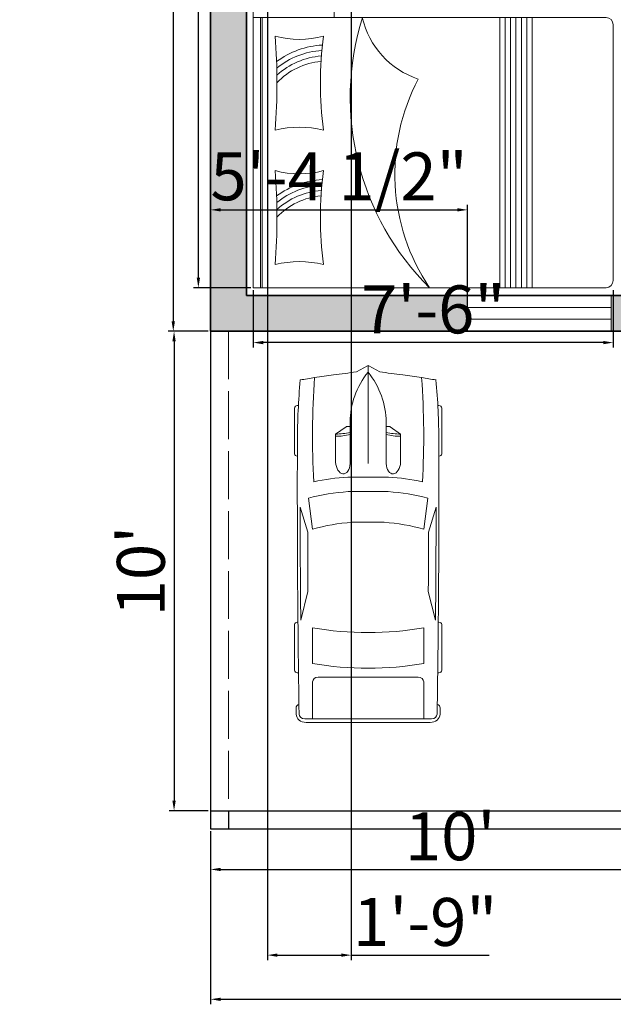
# Model space of a CAD drawing. Units: inches. Extents: x 1810 to 2254, y 313 to 1026.
# Tile 1 of 7: x 1828 to 1976, y 313 to 559. Entities that reach past the tile are written whole.
import ezdxf

# ---------------------------------------------------------------- set-up
doc = ezdxf.new("R2010")
doc.units = ezdxf.units.IN
doc.linetypes.add('ACAD_ISO02W100', pattern=[15, 12, -3])
for name, color, linetype, lineweight in [('A-ANNO-DIMS', 2, 'Continuous', 18), ('A-FURN', 8, 'Continuous', 18), ('A-GLAZ', 4, 'Continuous', 18), ('A-WALL', 7, 'Continuous', 35), ('C-PRKG-VEHC', 8, 'Continuous', 13), ('C-SITE', 7, 'Continuous', 25), ('C-SITE-HIDN', 7, 'ACAD_ISO02W100', 18)]:
    doc.layers.add(name, color=color, linetype=linetype, lineweight=lineweight)
doc.layers.add('A-WALL-PATT', color=252, linetype='Continuous', lineweight=13, true_color=0x939598)
doc.styles.get("Standard").update_dxf_attribs({"font": 'arial.ttf'})
doc.dimstyles.new('ISO-25', dxfattribs={"dimtxt": 12, "dimasz": 2.5, "dimexe": 1.25, "dimexo": 0.625, "dimtad": 1, "dimdec": 1, "dimlunit": 4, "dimtxsty": 'Standard', "dimcen": 2.5, "dimadec": 0, "dimazin": 0, "dimtfac": 1, "dimtdec": 1, "dimtmove": 0, "dimatfit": 3, "dimfxl": 1, "dimarcsym": 0})

# ---------------------------------------------------------------- blocks, each defined once
blk = doc.blocks.new('A$C50CC761E')
for p, q in [((0, 2), (0, 0.04)), ((0, 2), (1.5, 2)), ((1.5, 2), (1.5, 0.04)), ((0, 1.96), (1.5, 1.96)), ((0, 1.95), (1.5, 1.95)), ((0, 0.63), (1.5, 0.63)), ((0, 0.6), (1.5, 0.6)), ((0, 0.57), (1.5, 0.57)), ((0, 0.54), (1.5, 0.54)), ((0, 0.51), (1.5, 0.51)), ((0, 0.48), (1.5, 0.48)), ((0, 0.45), (1.5, 0.45)), ((1.46, 0), (0.04, 0))]:
    blk.add_line(p, q)
at = {"ltscale": 250}
for p, q in [((1.5, 2), (2.0303, 2)), ((2.0303, 2), (2.0303, 1.5501)), ((1.763, 1.8176), (1.763, 1.9295)), ((1.613, 1.7795), (1.7249, 1.7795)), ((1.8011, 1.7795), (1.913, 1.7795)), ((1.763, 1.6295), (1.763, 1.7414)), ((1.5, 1.5501), (2.0303, 1.5501))]:
    blk.add_line(p, q, dxfattribs=at)
for radius in [0.12, 0.0381]:
    blk.add_circle((1.763, 1.7795), radius, dxfattribs=at)
for centre, radius, start, end in [((0.3894, 5.1577), 3.2899, 265.4501, 274.5499), ((-0.4158, 1.744), 0.5605, 346.15, 13.85), ((0.1321, 1.5916), 0.3789, 4.7708, 46.8165), ((0.1321, 1.5916), 0.4089, 4.1373, 42.5614), ((0.1321, 1.5916), 0.4389, 3.5318, 39.1874), ((0.1321, 1.5916), 0.4689, 2.9489, 36.4321), ((1.1324, 1.744), 0.5004, 164.4468, 195.5532), ((1.1357, 5.1577), 3.2899, 265.4501, 274.5499), ((0.3306, 1.744), 0.5605, 346.15, 13.85), ((0.8784, 1.5916), 0.3789, 4.7708, 46.8165), ((0.8784, 1.5916), 0.4089, 4.1373, 42.5614), ((0.8784, 1.5916), 0.4389, 3.5318, 39.1874), ((0.8784, 1.5916), 0.4689, 2.9489, 36.4321), ((1.8788, 1.744), 0.5004, 164.4468, 195.5532), ((0.3894, -0.4129), 2.0395, 82.6483, 97.3517), ((1.1357, -0.4129), 2.0395, 82.6483, 97.3517), ((1.0573, -0.0269), 1.4879, 72.6898, 135.2822), ((1.6044, 0.9359), 0.4695, 102.8515, 161.769), ((0.6316, 0.0846), 1.1287, 62.1724, 124.0295), ((0.04, 0.04), 0.04, 180, 270), ((1.46, 0.04), 0.04, 270, 0)]:
    blk.add_arc(centre, radius, start, end)
blk = doc.blocks.new('*U14')
for p, q in [((21.1, 37.41), (21.1, 36.83)), ((46.55, 38.89), (22.35, 38.89)), ((47.8, 37.39), (47.8, 37.41)), ((135.45, 37.07), (135.45, 37.41)), ((136.7, 38.89), (160.9, 38.89)), ((162.15, 37.41), (162.15, 36.77)), ((70.03, 31.54), (86.41, 29.35)), ((87.99, 31.87), (74.76, 35.92)), ((134.31, 35.6), (119.29, 31.78)), ((186.47, -33.5), (186.47, 33.5)), ((188.4, -32.76), (188.4, 32.76)), ((138.42, 29.35), (157.25, 29.35)), ((164.52, 26.39), (164.52, -26.39)), ((186.47, 29.35), (167.01, 29.35)), ((32.27, 11.63), (36.13, 17.17)), ((36.13, 17.17), (50.94, 17.17)), ((32.12, 9.51), (32.12, 11.15)), ((58.92, -10.77), (58.92, 10.77)), ((66.55, -10.53), (66.55, 10.53)), ((186.47, -10.53), (186.47, 10.53)), ((3.27, 6.13), (0.1, 0.41)), ((29.77, 9.51), (51.68, 9.51)), ((82.74, 8.5), (82.74, -8.5)), ((0, 0), (51.68, 0)), ((0.1, -0.41), (3.27, -6.13)), ((29.77, -9.51), (51.68, -9.51)), ((32.12, -9.51), (32.12, -11.15)), ((32.27, -11.63), (36.13, -17.17)), ((36.13, -17.17), (50.94, -17.17)), ((86.41, -29.35), (70.03, -31.54)), ((157.25, -29.35), (138.42, -29.35)), ((167.01, -29.35), (186.47, -29.35)), ((87.99, -31.87), (74.76, -35.92)), ((134.31, -35.6), (119.29, -31.78)), ((21.1, -37.41), (21.1, -36.83)), ((46.55, -38.89), (22.35, -38.89)), ((47.8, -37.39), (47.8, -37.41)), ((135.45, -37.07), (135.45, -37.41)), ((136.7, -38.89), (160.9, -38.89)), ((162.15, -37.41), (162.15, -36.77))]:
    blk.add_line(p, q)
for centre, major_axis, ratio, start_param, end_param in [((41.19, -490.86), (0, 528.23), 0.842304, 0.00281, 0.075598), ((22.35, 37.41), (0, -1.48), 0.842304, 3.141593, 4.712389), ((64.48, -10555.62), (0, 10593.03), 0.842304, -0.013397, 0.002797), ((46.55, 37.41), (0, 1.48), 0.842304, -1.570796, 0), ((136.7, 37.41), (0, -1.48), 0.842304, 3.141593, 4.712389), ((160.9, 37.41), (0, 1.48), 0.842304, -1.570796, 0), ((180.63, 35.84), (0, 2.22), 0.842304, -0.013017, 1.249894), ((64.48, -10556.36), (0, 10595.31), 0.842304, -0.013397, -0.013017), ((183.98, 33.5), (0, -2.96), 0.842304, 1.570796, 3.128196), ((183.98, 32.76), (0, -5.25), 0.842304, 1.570796, 3.128196), ((266.03, -27.52), (0, 313.31), 0.842304, 1.367076, 1.39176), ((135.29, 5.39), (0, 81.77), 0.842304, 1.245306, 1.50788), ((64.48, -10555.62), (0, -10591.55), 0.842304, 3.133765, 3.140441), ((95.79, -3666.35), (0, -3698.24), 0.842304, 3.134049, 3.144098), ((259.18, -27.52), (0, -305.3), 0.842304, 4.528606, 4.561838), ((37.47, -593.96), (0, -623.33), 0.842304, 3.096046, 3.200911), ((134.4, 5.39), (0, -89.78), 0.842304, 4.449482, 4.652344), ((149.6, 2.8), (0, -79.58), 0.842304, 4.372215, 4.640744), ((17.08, 0), (0, 147.02), 0.842304, 4.511394, 4.913384), ((35.91, 0), (0, 147.02), 0.842304, 4.511394, 4.913384), ((167.01, 26.39), (0, 2.96), 0.842304, 0, 1.570796), ((-204.49, 52.4), (0, -250.96), 0.842304, 1.385369, 1.434372), ((13.04, 17.01), (0, 27.42), 0.842304, 4.435146, 4.718221), ((14.2, 17.01), (0, 27.42), 0.842304, 4.435146, 4.718221), ((50.79, 13.34), (6.34, -0.36), 0.603834, -1.395552, 1.581315), ((32.75, 11.15), (0, 0.74), 0.842304, 0.879714, 1.570796), ((29.77, -46.66), (0, 56.17), 0.842304, 0, 0.590319), ((0.62, 0), (0, -0.74), 0.842304, 4.131459, 5.293319), ((29.77, 46.66), (0, 56.17), 0.842304, 2.551274, 3.141593), ((-204.49, -52.4), (0, 250.96), 0.842304, -1.434372, -1.385369), ((13.04, -17.01), (0, -27.42), 0.842304, 1.564964, 1.848039), ((14.2, -17.01), (0, -27.42), 0.842304, 1.564964, 1.848039), ((149.6, -2.8), (0, -79.58), 0.842304, -1.499151, -1.230623), ((32.75, -11.15), (0, -0.74), 0.842304, 4.712389, 5.403472), ((134.4, -5.39), (0, -89.78), 0.842304, -1.510751, -1.307889), ((135.29, -5.39), (0, -81.77), 0.842304, -1.50788, -1.245306), ((259.18, 27.52), (0, 305.3), 0.842304, 1.721348, 1.754579), ((266.03, 27.52), (0, 313.31), 0.842304, 1.749832, 1.774517), ((37.47, 593.96), (0, -623.33), 0.842304, -0.059319, 0.045547), ((167.01, -26.39), (0, -2.96), 0.842304, 4.712389, 6.283185), ((41.19, 490.86), (0, -528.23), 0.842304, -0.075598, -0.00281), ((64.48, 10555.62), (0, -10591.55), 0.842304, 0.001152, 0.007828), ((95.79, 3666.35), (0, -3698.24), 0.842304, -0.002505, 0.007544), ((183.98, -33.5), (0, 2.96), 0.842304, 3.15499, 4.712389), ((183.98, -32.76), (0, -5.25), 0.842304, 0.013397, 1.570796), ((22.35, -37.41), (0, 1.48), 0.842304, 1.570796, 3.141593), ((64.48, 10555.62), (0, 10593.03), 0.842304, 3.138796, 3.15499), ((46.55, -37.41), (0, -1.48), 0.842304, 0, 1.570796), ((136.7, -37.41), (0, -1.48), 0.842304, -1.570796, 0), ((160.9, -37.41), (0, 1.48), 0.842304, 3.141593, 4.712389), ((180.63, -35.84), (0, -2.22), 0.842304, -1.249894, 0.013017), ((64.48, 10556.36), (0, 10595.31), 0.842304, 3.15461, 3.15499)]:
    blk.add_ellipse(centre, major_axis=major_axis, ratio=ratio, start_param=start_param, end_param=end_param)
at = {"extrusion": (0, 0, -1)}
blk.add_ellipse((50.79, -13.34), major_axis=(6.34, 0.36), ratio=0.603834, start_param=-1.395552, end_param=1.581315, dxfattribs=at)
blk = doc.blocks.new('*D24')
at = {"layer": 'A-ANNO-DIMS', "color": 0, "lineweight": -2, "transparency": 16777216}
for p, q in [((1874.74, 481.11), (1864.94, 481.11)), ((1866.19, 478.61), (1866.19, 363.61)), ((1874.74, 361.11), (1864.94, 361.11))]:
    blk.add_line(p, q, dxfattribs=at)
at = {"layer": 'A-ANNO-DIMS', "color": 0, "transparency": 16777216}
for points in [[(1865.77, 478.61), (1866.6, 478.61), (1866.19, 481.11)], [(1865.77, 363.61), (1866.6, 363.61), (1866.19, 361.11)]]:
    blk.add_solid(points, dxfattribs=at)
at = {"layer": 'Defpoints', "color": 0, "transparency": 16777216}
for p in [(1875.36, 481.11), (1866.19, 361.11), (1875.36, 361.11)]:
    blk.add_point(p, dxfattribs=at)
at = {"layer": 'A-ANNO-DIMS', "color": 0, "transparency": 16777216, "insert": (1859.43, 421.11), "char_height": 12, "attachment_point": 5, "rotation": 90}
blk.add_mtext("10'", dxfattribs=at)
blk = doc.blocks.new('*D25')
at = {"layer": 'A-ANNO-DIMS', "color": 0, "lineweight": -2, "transparency": 16777216}
for p, q in [((1874.74, 860.61), (1864.75, 860.61)), ((1866, 858.11), (1866, 483.61)), ((1874.74, 481.11), (1864.75, 481.11))]:
    blk.add_line(p, q, dxfattribs=at)
at = {"layer": 'A-ANNO-DIMS', "color": 0, "transparency": 16777216}
for points in [[(1865.58, 858.11), (1866.42, 858.11), (1866, 860.61)], [(1865.58, 483.61), (1866.42, 483.61), (1866, 481.11)]]:
    blk.add_solid(points, dxfattribs=at)
at = {"layer": 'Defpoints', "color": 0, "transparency": 16777216}
for p in [(1875.36, 860.61), (1866, 481.11), (1875.36, 481.11)]:
    blk.add_point(p, dxfattribs=at)
at = {"layer": 'A-ANNO-DIMS', "color": 0, "transparency": 16777216, "insert": (1851.22, 670.86), "char_height": 12, "attachment_point": 5, "rotation": 90}
blk.add_mtext('31\'-7{\\H1x;\\S1/2;}"', dxfattribs=at)
blk = doc.blocks.new('*D26')
at = {"layer": 'A-ANNO-DIMS', "color": 0, "lineweight": -2, "transparency": 16777216}
for p, q in [((1875.36, 355.99), (1875.36, 312.66)), ((2139.36, 355.99), (2139.36, 312.66)), ((1877.86, 313.91), (2136.86, 313.91))]:
    blk.add_line(p, q, dxfattribs=at)
at = {"layer": 'A-ANNO-DIMS', "color": 0, "transparency": 16777216}
for points in [[(1877.86, 314.32), (1877.86, 313.49), (1875.36, 313.91)], [(2136.86, 314.32), (2136.86, 313.49), (2139.36, 313.91)]]:
    blk.add_solid(points, dxfattribs=at)
at = {"layer": 'Defpoints', "color": 0, "transparency": 16777216}
for p in [(1875.36, 356.61), (2139.36, 356.61), (2139.36, 313.91)]:
    blk.add_point(p, dxfattribs=at)
at = {"layer": 'A-ANNO-DIMS', "color": 0, "transparency": 16777216, "insert": (2007.36, 320.55), "char_height": 12, "attachment_point": 5}
blk.add_mtext("22'", dxfattribs=at)
blk = doc.blocks.new('*D27')
at = {"layer": 'A-ANNO-DIMS', "color": 0, "lineweight": -2, "transparency": 16777216}
for p, q in [((1875.36, 355.99), (1875.36, 345.16)), ((1995.39, 355.99), (1995.39, 345.16)), ((1877.86, 346.41), (1992.89, 346.41))]:
    blk.add_line(p, q, dxfattribs=at)
at = {"layer": 'A-ANNO-DIMS', "color": 0, "transparency": 16777216}
for points in [[(1877.86, 346.82), (1877.86, 345.99), (1875.36, 346.41)], [(1992.89, 346.82), (1992.89, 345.99), (1995.39, 346.41)]]:
    blk.add_solid(points, dxfattribs=at)
at = {"layer": 'Defpoints', "color": 0, "transparency": 16777216}
for p in [(1875.36, 356.61), (1995.39, 356.61), (1995.39, 346.41)]:
    blk.add_point(p, dxfattribs=at)
at = {"layer": 'A-ANNO-DIMS', "color": 0, "transparency": 16777216, "insert": (1935.38, 353.16), "char_height": 12, "attachment_point": 5}
blk.add_mtext("10'", dxfattribs=at)
blk = doc.blocks.new('WIN-36IN-WALL9')
for p, q in [((0, 9), (0, 0)), ((36, 9), (36, 0)), ((0, 6), (36, 6)), ((0, 3), (36, 3))]:
    blk.add_line(p, q)
blk = doc.blocks.new('*D38')
at = {"layer": 'A-ANNO-DIMS', "color": 0, "lineweight": -2, "transparency": 16777216}
for p, q in [((1872.28, 583.59), (1872.28, 751.92)), ((1885.39, 583.59), (1871.03, 583.59)), ((1872.28, 494.52), (1872.28, 581.09)), ((1885.39, 492.02), (1871.03, 492.02))]:
    blk.add_line(p, q, dxfattribs=at)
at = {"layer": 'A-ANNO-DIMS', "color": 0, "transparency": 16777216}
for points in [[(1871.87, 581.09), (1872.7, 581.09), (1872.28, 583.59)], [(1871.87, 494.52), (1872.7, 494.52), (1872.28, 492.02)]]:
    blk.add_solid(points, dxfattribs=at)
at = {"layer": 'Defpoints', "color": 0, "transparency": 16777216}
for p in [(1872.28, 583.59), (1886.02, 583.59), (1886.02, 492.02)]:
    blk.add_point(p, dxfattribs=at)
at = {"layer": 'A-ANNO-DIMS', "color": 0, "transparency": 16777216, "insert": (1865.45, 669.01), "char_height": 12, "attachment_point": 5, "rotation": 90}
blk.add_mtext('BED GROUP 7\'-7 1/2"', dxfattribs=at)
blk = doc.blocks.new('*D39')
at = {"layer": 'A-ANNO-DIMS', "color": 0, "lineweight": -2, "transparency": 16777216}
for p, q in [((1886.02, 491.4), (1886.02, 477.04)), ((1976.21, 491.4), (1976.21, 477.04)), ((1973.71, 478.29), (1888.52, 478.29))]:
    blk.add_line(p, q, dxfattribs=at)
at = {"layer": 'A-ANNO-DIMS', "color": 0, "transparency": 16777216}
for points in [[(1888.52, 478.71), (1888.52, 477.87), (1886.02, 478.29)], [(1973.71, 478.71), (1973.71, 477.87), (1976.21, 478.29)]]:
    blk.add_solid(points, dxfattribs=at)
at = {"layer": 'Defpoints', "color": 0, "transparency": 16777216}
for p in [(1886.02, 492.02), (1976.21, 492.02), (1886.02, 478.29)]:
    blk.add_point(p, dxfattribs=at)
at = {"layer": 'A-ANNO-DIMS', "color": 0, "transparency": 16777216, "insert": (1931.11, 485.04), "char_height": 12, "attachment_point": 5}
blk.add_mtext('7\'-6"', dxfattribs=at)
blk = doc.blocks.new('*D53')
at = {"layer": 'A-ANNO-DIMS', "color": 0, "lineweight": -2, "transparency": 16777216}
for p, q in [((1875.36, 481.74), (1875.36, 512.76)), ((1939.68, 481.74), (1939.68, 512.76)), ((1877.86, 511.51), (1937.18, 511.51))]:
    blk.add_line(p, q, dxfattribs=at)
at = {"layer": 'A-ANNO-DIMS', "color": 0, "transparency": 16777216}
for points in [[(1877.86, 511.93), (1877.86, 511.1), (1875.36, 511.51)], [(1937.18, 511.93), (1937.18, 511.1), (1939.68, 511.51)]]:
    blk.add_solid(points, dxfattribs=at)
at = {"layer": 'Defpoints', "color": 0, "transparency": 16777216}
for p in [(1939.68, 511.51), (1875.36, 481.11), (1939.68, 481.11)]:
    blk.add_point(p, dxfattribs=at)
at = {"layer": 'A-ANNO-DIMS', "color": 0, "transparency": 16777216, "insert": (1907.52, 518.34), "char_height": 12, "attachment_point": 5}
blk.add_mtext('5\'-4 1/2"', dxfattribs=at)
blk = doc.blocks.new('*D72')
at = {"layer": 'A-ANNO-DIMS', "color": 0, "lineweight": -2, "transparency": 16777216}
for p, q in [((1889.6, 613.99), (1889.6, 323.71)), ((1910.6, 613.99), (1910.6, 323.71)), ((1892.1, 324.96), (1908.1, 324.96)), ((1910.6, 324.96), (1945.12, 324.96))]:
    blk.add_line(p, q, dxfattribs=at)
at = {"layer": 'A-ANNO-DIMS', "color": 0, "transparency": 16777216}
for points in [[(1892.1, 325.38), (1892.1, 324.55), (1889.6, 324.96)], [(1908.1, 325.38), (1908.1, 324.55), (1910.6, 324.96)]]:
    blk.add_solid(points, dxfattribs=at)
at = {"layer": 'Defpoints', "color": 0, "transparency": 16777216}
for p in [(1889.6, 614.61), (1910.6, 614.61), (1910.6, 324.96)]:
    blk.add_point(p, dxfattribs=at)
at = {"layer": 'A-ANNO-DIMS', "color": 0, "transparency": 16777216, "insert": (1929.11, 331.72), "char_height": 12, "attachment_point": 5}
blk.add_mtext('1\'-9"', dxfattribs=at)

msp = doc.modelspace()

# ---------------------------------------------------------------- hatches: boundary and pattern name
at = {"layer": 'A-WALL-PATT'}
h = msp.add_hatch(color=256, dxfattribs=at)
h.dxf.hatch_style = 1
h.paths.add_polyline_path([(1943.78, 860.61), (1875.36, 860.61), (1875.36, 706.11), (1884.36, 706.11), (1884.36, 715.11), (1968.36, 715.11), (1968.36, 703.36), (1971.96, 703.36), (1972.86, 703.36), (1972.86, 715.11), (1976.68, 715.11), (1976.68, 719.61), (1884.36, 719.61), (1884.36, 851.61), (1943.73, 851.61)])
h.paths.add_polyline_path([(2048.15, 860.61), (1979.78, 860.61), (1979.73, 851.61), (2016.36, 851.61), (2016.36, 719.61), (2012.68, 719.61), (2012.68, 716.01), (2012.68, 715.11), (2024.44, 715.11), (2024.44, 719.61), (2020.86, 719.61), (2020.86, 851.61), (2048.15, 851.61)])
h.paths.add_polyline_path([(2139.36, 860.61), (2084.15, 860.61), (2084.15, 851.61), (2130.36, 851.61), (2130.36, 719.61), (2060.44, 719.61), (2060.44, 716.01), (2060.44, 715.11), (2130.36, 715.11), (2130.36, 673.52), (2139.36, 673.52)])
h.paths.add_polyline_path([(1884.36, 682.11), (1875.36, 682.11), (1875.36, 654.79), (1884.36, 654.79), (1884.36, 662.61), (1968.36, 662.61), (1968.36, 647.42), (1971.96, 647.42), (1972.86, 647.42), (1972.86, 679.36), (1968.36, 679.36), (1968.36, 667.11), (1884.36, 667.11)])
h.paths.add_polyline_path([(1884.36, 610.11), (1972.86, 610.11), (1976.27, 610.11), (1976.27, 614.61), (1972.86, 614.61), (1972.86, 623.42), (1968.36, 623.42), (1968.36, 614.61), (1884.36, 614.61), (1884.36, 630.79), (1875.36, 630.79), (1875.36, 481.11), (1939.68, 481.11), (1939.68, 490.11), (1884.36, 490.11)])
h.paths.add_polyline_path([(2007.36, 518.61), (2038.86, 518.61), (2038.86, 494.59), (2043.36, 494.59), (2043.36, 518.61), (2070.36, 518.61), (2070.36, 523.11), (2007.36, 523.11), (2007.36, 614.61), (2000.27, 614.61), (2000.27, 610.11), (2003.36, 610.11), (2003.36, 490.11), (1975.68, 490.11), (1975.68, 481.11), (2007.36, 481.11)])
h.paths.add_polyline_path([(2139.36, 637.52), (2130.36, 637.52), (2130.36, 434.61), (2043.36, 434.61), (2043.36, 458.59), (2038.86, 458.59), (2038.86, 434.61), (2035.41, 434.61), (2035.41, 431.01), (2035.41, 425.61), (2139.36, 425.61)])

# ---------------------------------------------------------------- linework, layer by layer
at = {"layer": 'A-WALL'}
for p, q in [((1875.36, 860.61), (1875.36, 481.11)), ((1884.36, 610.11), (1884.36, 490.11)), ((1884.36, 490.11), (2003.36, 490.11)), ((1875.36, 481.11), (2007.36, 481.11))]:
    msp.add_line(p, q, dxfattribs=at)
at = {"layer": 'C-SITE'}
for p, q in [((1875.36, 481.11), (1875.36, 356.61)), ((1875.36, 361.11), (1991.39, 361.11)), ((1879.86, 361.11), (1879.86, 356.61)), ((1875.36, 356.61), (1995.39, 356.61))]:
    msp.add_line(p, q, dxfattribs=at)
at = {"layer": 'C-SITE-HIDN'}
msp.add_line((1879.86, 481.11), (1879.86, 361.11), dxfattribs=at)

# ---------------------------------------------------------------- block references
at = {"layer": 'A-FURN', "xscale": 45.09822183510779, "yscale": 45.09822183510779, "zscale": 45.09822183510779, "rotation": 90}
msp.add_blockref('A$C50CC761E', (1976.21, 492.02), dxfattribs=at)
at = {"layer": 'A-GLAZ'}
msp.add_blockref('WIN-36IN-WALL9', (1939.68, 481.11), dxfattribs=at)
at = {"layer": 'C-PRKG-VEHC', "xscale": 0.4741609533567669, "yscale": 0.4741609533567669, "zscale": 0.4741609533567669, "rotation": 270}
msp.add_blockref('*U14', (1914.81, 472.53), dxfattribs=at)

# ---------------------------------------------------------------- dimensions: what is measured, and where the dimension line sits
at = {"layer": 'A-ANNO-DIMS'}
for base, p1, p2, angle, override, picture, middle in [((1866, 481.11), (1875.36, 860.61), (1875.36, 481.11), 90, {"dimclrd": 0, "dimclre": 0, "dimclrt": 0}, '*D25', (1851.22, 670.86)), ((1939.68, 511.51), (1875.36, 481.11), (1939.68, 481.11), 0, {"dimdec": 1, "dimlfac": 1, "dimrnd": 0, "dimzin": 1, "dimdsep": 46, "dimlunit": 4, "dimfrac": 2}, '*D53', (1907.52, 518.34)), ((1886.02, 478.29), (1976.21, 492.02), (1886.02, 492.02), 180, {"dimdec": 1, "dimlfac": 1, "dimrnd": 0, "dimzin": 1, "dimdsep": 46, "dimlunit": 4, "dimfrac": 2}, '*D39', (1931.11, 485.04)), ((1866.19, 361.11), (1875.36, 481.11), (1875.36, 361.11), 90, {"dimclrd": 0, "dimclre": 0, "dimclrt": 0}, '*D24', (1859.43, 421.11))]:
    dim = msp.add_linear_dim(base=base, p1=p1, p2=p2, angle=angle, dimstyle='ISO-25', override=override, dxfattribs=at)
    dim.commit()
    dim.dimension.update_dxf_attribs({"geometry": picture, "text_midpoint": middle})
dim = msp.add_linear_dim(base=(1872.28, 583.59), p1=(1886.02, 492.02), p2=(1886.02, 583.59), angle=90, text='BED GROUP <>', dimstyle='ISO-25', override={"dimdec": 1, "dimlfac": 1, "dimrnd": 0, "dimzin": 1, "dimdsep": 46, "dimlunit": 4, "dimfrac": 2}, dxfattribs=at)
dim.commit()
dim.dimension.update_dxf_attribs({"geometry": '*D38', "text_midpoint": (1865.45, 669.01)})
for base, p1, p2, override, picture, middle in [((1910.6, 324.96), (1889.6, 614.61), (1910.6, 614.61), {"dimdec": 1, "dimlfac": 1, "dimrnd": 0, "dimzin": 1, "dimdsep": 46, "dimlunit": 4, "dimfrac": 2}, '*D72', (1929.11, 331.72)), ((1995.39, 346.41), (1875.36, 356.61), (1995.39, 356.61), {"dimclrd": 0, "dimclre": 0, "dimclrt": 0}, '*D27', (1935.38, 353.16)), ((2139.36, 313.91), (1875.36, 356.61), (2139.36, 356.61), {"dimclrd": 0, "dimclre": 0, "dimclrt": 0}, '*D26', (2007.36, 320.55))]:
    dim = msp.add_linear_dim(base=base, p1=p1, p2=p2, dimstyle='ISO-25', override=override, dxfattribs=at)
    dim.commit()
    dim.dimension.update_dxf_attribs({"geometry": picture, "text_midpoint": middle})

doc.saveas('drawing.dxf')
